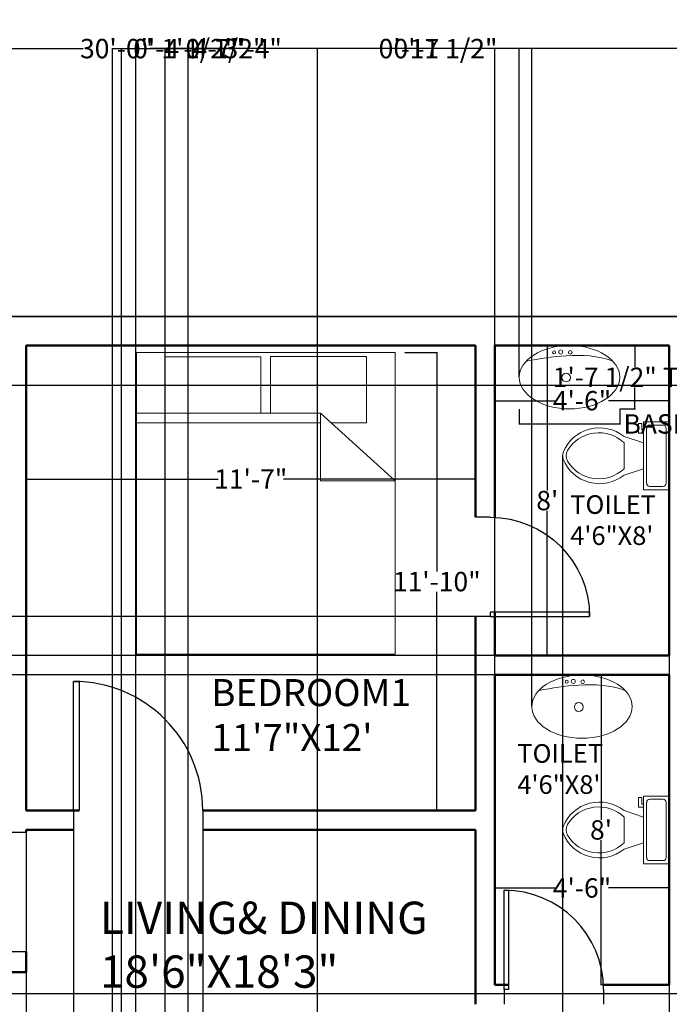
# Model space of a CAD drawing. Units: inches. Extents: x -56 to 545, y -536 to 185.
# Tile 6 of 7: x 144 to 345, y -120 to 185. Entities that reach past the tile are written whole.
import ezdxf

# ---------------------------------------------------------------- set-up
doc = ezdxf.new("R2010")
doc.units = ezdxf.units.IN
doc.header["$MEASUREMENT"] = 0
for name, color, linetype, lineweight in [('A-ANNO-DIMS', 2, 'Continuous', 18), ('A-AREA-IDEN', 4, 'Continuous', 25), ('A-DOOR', 4, 'Continuous', 25), ('A-FLOR-FIXT', 8, 'Continuous', 18), ('A-FURN', 8, 'Continuous', 18), ('A-WALL', 7, 'Continuous', 50), ('C-PROP', 7, 'Continuous', 35)]:
    doc.layers.add(name, color=color, linetype=linetype, lineweight=lineweight)
doc.styles.get("Standard").update_dxf_attribs({"font": 'arial.ttf'})
doc.dimstyles.get("Standard").update_dxf_attribs({"dimtxt": 6, "dimasz": 0.18, "dimexe": 0.18, "dimexo": 0.0625, "dimgap": 0.09, "dimtad": 0, "dimtih": 1, "dimtoh": 1, "dimdec": 0, "dimzin": 0, "dimdsep": 46, "dimlunit": 3, "dimtxsty": 'Standard', "dimcen": 0.09, "dimclrd": 3, "dimclre": 3, "dimclrt": 3, "dimadec": 0, "dimazin": 0, "dimtfac": 1, "dimtdec": 0, "dimtofl": 0, "dimtmove": 0, "dimatfit": 3, "dimfxl": 1, "dimtolj": 1, "dimtzin": 0, "dimarcsym": 0})

# ---------------------------------------------------------------- blocks, each defined once
blk = doc.blocks.new('CAMAKING')
for points in [[(0.8635, 0), (-0.8635, 0)], [(-0.8635, -2.0147), (-0.8635, 0)], [(0.8635, 0), (0.8635, -2.0147)], [(-0.6723, -0.4077), (-0.6723, -0.0281)], [(-0.6723, -0.0281), (-0.0328, -0.0281)], [(-0.0328, -0.0281), (-0.0328, -0.4077)], [(0.6716, -0.027), (0.0319, -0.027)], [(0.0319, -0.027), (0.0319, -0.4077)], [(0.6716, -0.4686), (0.6716, -0.027)], [(0.3645, -0.4056), (-0.8635, -0.4056)], [(0.8635, -0.857), (0.3645, -0.4056)], [(0.3645, -0.4702), (0.3645, -0.4056)], [(-0.8635, -0.4702), (0.3645, -0.4702)], [(0.3645, -0.4702), (0.3645, -0.857)], [(0.4362, -0.4686), (0.6716, -0.4686)], [(0.3645, -0.857), (0.8635, -0.857)], [(0.8635, -2.0147), (-0.8635, -2.0147)]]:
    blk.add_lwpolyline(points)
blk = doc.blocks.new('*U5')
for p, q in [((9.5, -6), (9.5, -2)), ((-10, -8.5), (-8, -8.5)), ((-10, -9.5), (-10, -8.5)), ((-8, -8.5), (-8, -8)), ((-7, -8), (-7, -9.5)), ((-4, -8), (-6, -14)), ((4, -8), (6, -14)), ((-7, -9.5), (-10, -9.5)), ((4, -14), (-4, -14))]:
    blk.add_line(p, q)
blk.add_lwpolyline([(10.5, -8), (10.5, 0), (-10.5, 0), (-10.5, -8)], close=True)
for points in [[(-9.5, -2), (-9.5, -6)], [(8.5, -1), (-8.5, -1)], [(-8.5, -7), (8.5, -7)]]:
    blk.add_lwpolyline(points)
for centre, radius, start, end in [((-8.62, -1.88), 0.884, 81.8699, 188.1301), ((8.62, -1.88), 0.884, 351.8699, 98.1301), ((-8.62, -6.12), 0.884, 171.8699, 278.1301), ((8.62, -6.12), 0.884, 261.8699, 8.1301), ((3.52, -21.58), 12.17, 141.4691, 247.9714), ((4.2, -21.82), 11.33, 136.3677, 238.9468), ((-3.52, -21.58), 12.17, 292.0284, 38.5307), ((-4.2, -21.82), 11.33, 301.053, 43.6321), ((0, -27.88), 4, 245.7318, 294.2682), ((0, -29), 4, 254.8605, 285.1395)]:
    blk.add_arc(centre, radius, start, end)
blk = doc.blocks.new('*U7')
for p, q in [((0, 0), (0, -6)), ((40, 0), (40, -6))]:
    blk.add_line(p, q)
blk.add_lwpolyline([(0, 0), (0, 40), (1.75, 40), (1.75, 0)], close=True)
blk.add_arc((0, 0), 40, 0, 90)
blk = doc.blocks.new('*D26')
at = {"layer": 'A-ANNO-DIMS', "color": 0, "lineweight": -2, "transparency": 16777216}
for p, q in [((146.03, 50.03), (146.03, 42.62)), ((285.03, 50.03), (285.03, 42.62)), ((146.21, 42.8), (205.42, 42.8)), ((284.85, 42.8), (225.65, 42.8))]:
    blk.add_line(p, q, dxfattribs=at)
at = {"layer": 'A-ANNO-DIMS', "color": 0, "transparency": 16777216}
for points in [[(146.21, 42.83), (146.21, 42.77), (146.03, 42.8)], [(284.85, 42.83), (284.85, 42.77), (285.03, 42.8)]]:
    blk.add_solid(points, dxfattribs=at)
at = {"layer": 'Defpoints', "color": 0, "transparency": 16777216}
for p in [(146.03, 50.1), (285.03, 50.1), (285.03, 42.8)]:
    blk.add_point(p, dxfattribs=at)
at = {"layer": 'A-ANNO-DIMS', "color": 0, "transparency": 16777216, "insert": (215.53, 42.8), "char_height": 6, "attachment_point": 5}
blk.add_mtext('\\A1;11\'-7"', dxfattribs=at)
blk = doc.blocks.new('*D27')
at = {"layer": 'A-ANNO-DIMS', "color": 0, "lineweight": -2, "transparency": 16777216}
for p, q in [((263.2, 81.99), (273.28, 81.99)), ((273.1, 81.81), (273.1, 14.23)), ((273.1, -59.66), (273.1, 7.92)), ((263.2, -59.84), (273.28, -59.84))]:
    blk.add_line(p, q, dxfattribs=at)
at = {"layer": 'A-ANNO-DIMS', "color": 0, "transparency": 16777216}
for points in [[(273.07, 81.81), (273.13, 81.81), (273.1, 81.99)], [(273.07, -59.66), (273.13, -59.66), (273.1, -59.84)]]:
    blk.add_solid(points, dxfattribs=at)
at = {"layer": 'Defpoints', "color": 0, "transparency": 16777216}
for p in [(263.14, 81.99), (273.1, 81.99), (263.14, -59.84)]:
    blk.add_point(p, dxfattribs=at)
at = {"layer": 'A-ANNO-DIMS', "color": 0, "transparency": 16777216, "insert": (273.1, 11.07), "char_height": 6, "attachment_point": 5}
blk.add_mtext('\\A1;11\'-10"', dxfattribs=at)
blk = doc.blocks.new('*D28')
at = {"layer": 'A-ANNO-DIMS', "color": 0, "lineweight": -2, "transparency": 16777216}
for p, q in [((291.03, 50.82), (291.03, 67.26)), ((291.21, 67.08), (309.85, 67.08)), ((344.85, 67.08), (326.22, 67.08)), ((345.03, 50.09), (345.03, 67.26))]:
    blk.add_line(p, q, dxfattribs=at)
at = {"layer": 'A-ANNO-DIMS', "color": 0, "transparency": 16777216}
for points in [[(291.21, 67.11), (291.21, 67.05), (291.03, 67.08)], [(344.85, 67.11), (344.85, 67.05), (345.03, 67.08)]]:
    blk.add_solid(points, dxfattribs=at)
at = {"layer": 'Defpoints', "color": 0, "transparency": 16777216}
for p in [(345.03, 67.08), (291.03, 50.76), (345.03, 50.03)]:
    blk.add_point(p, dxfattribs=at)
at = {"layer": 'A-ANNO-DIMS', "color": 0, "transparency": 16777216, "insert": (318.03, 67.08), "char_height": 6, "attachment_point": 5}
blk.add_mtext('\\A1;4\'-6"', dxfattribs=at)
blk = doc.blocks.new('*D29')
at = {"layer": 'A-ANNO-DIMS', "color": 0, "lineweight": -2, "transparency": 16777216}
for p, q in [((335.97, 84.16), (307.11, 84.16)), ((307.29, 83.98), (307.29, 39.31)), ((307.29, -11.66), (307.29, 33.01)), ((335.97, -11.84), (307.11, -11.84))]:
    blk.add_line(p, q, dxfattribs=at)
at = {"layer": 'A-ANNO-DIMS', "color": 0, "transparency": 16777216}
for points in [[(307.26, 83.98), (307.32, 83.98), (307.29, 84.16)], [(307.26, -11.66), (307.32, -11.66), (307.29, -11.84)]]:
    blk.add_solid(points, dxfattribs=at)
at = {"layer": 'Defpoints', "color": 0, "transparency": 16777216}
for p in [(336.04, 84.16), (307.29, -11.84), (336.04, -11.84)]:
    blk.add_point(p, dxfattribs=at)
at = {"layer": 'A-ANNO-DIMS', "color": 0, "transparency": 16777216, "insert": (307.29, 36.16), "char_height": 6, "attachment_point": 5}
blk.add_mtext("\\A1;8'", dxfattribs=at)
blk = doc.blocks.new('*D30')
at = {"layer": 'A-ANNO-DIMS', "color": 0, "lineweight": -2, "transparency": 16777216}
for p, q in [((291.03, -35.73), (291.03, -83.99)), ((345.03, -35.73), (345.03, -83.99)), ((291.21, -83.81), (309.85, -83.81)), ((344.85, -83.81), (326.22, -83.81))]:
    blk.add_line(p, q, dxfattribs=at)
at = {"layer": 'A-ANNO-DIMS', "color": 0, "transparency": 16777216}
for points in [[(291.21, -83.78), (291.21, -83.84), (291.03, -83.81)], [(344.85, -83.78), (344.85, -83.84), (345.03, -83.81)]]:
    blk.add_solid(points, dxfattribs=at)
at = {"layer": 'Defpoints', "color": 0, "transparency": 16777216}
for p in [(291.03, -35.67), (345.03, -35.67), (345.03, -83.81)]:
    blk.add_point(p, dxfattribs=at)
at = {"layer": 'A-ANNO-DIMS', "color": 0, "transparency": 16777216, "insert": (318.03, -83.81), "char_height": 6, "attachment_point": 5}
blk.add_mtext('\\A1;4\'-6"', dxfattribs=at)
blk = doc.blocks.new('*D31')
at = {"layer": 'A-ANNO-DIMS', "color": 0, "lineweight": -2, "transparency": 16777216}
for p, q in [((340.5, -17.84), (323.74, -17.84)), ((323.92, -18.02), (323.92, -62.69)), ((323.92, -113.66), (323.92, -68.99)), ((340.5, -113.84), (323.74, -113.84))]:
    blk.add_line(p, q, dxfattribs=at)
at = {"layer": 'A-ANNO-DIMS', "color": 0, "transparency": 16777216}
for points in [[(323.89, -18.02), (323.95, -18.02), (323.92, -17.84)], [(323.89, -113.66), (323.95, -113.66), (323.92, -113.84)]]:
    blk.add_solid(points, dxfattribs=at)
at = {"layer": 'Defpoints', "color": 0, "transparency": 16777216}
for p in [(340.57, -17.84), (323.92, -113.84), (340.57, -113.84)]:
    blk.add_point(p, dxfattribs=at)
at = {"layer": 'A-ANNO-DIMS', "color": 0, "transparency": 16777216, "insert": (323.92, -65.84), "char_height": 6, "attachment_point": 5}
blk.add_mtext("\\A1;8'", dxfattribs=at)
blk = doc.blocks.new('LAV-OVAL')
for centre, radius in [((-4.76, 7.71), 0.472), ((-2.71, 7.81), 0.633), ((0.21, 7.71), 0.565), ((-1.02, -0.12), 1.35)]:
    blk.add_circle(centre, radius)
blk.add_ellipse((0, 0), major_axis=(-15.53, 0), ratio=0.631418)
blk.add_open_spline([(-13.36, 5), (-9.28, 5.7), (-0.46, 7.23), (8.86, 6.68), (13.36, 5)], degree=3, knots=[0, 0, 0, 0, 12.471835, 26.932887, 26.932887, 26.932887, 26.932887])
blk = doc.blocks.new('*D39')
at = {"layer": 'A-ANNO-DIMS', "color": 3, "lineweight": -2, "transparency": 16777216}
for p, q in [((298.63, 64.49), (298.63, 59.71)), ((329.69, 64.49), (329.69, 59.71)), ((298.81, 59.89), (329.51, 59.89)), ((329.69, 59.89), (329.87, 59.89))]:
    blk.add_line(p, q, dxfattribs=at)
at = {"layer": 'A-ANNO-DIMS', "color": 3, "transparency": 16777216}
for points in [[(298.81, 59.92), (298.81, 59.86), (298.63, 59.89)], [(329.51, 59.92), (329.51, 59.86), (329.69, 59.89)]]:
    blk.add_solid(points, dxfattribs=at)
at = {"layer": 'Defpoints', "color": 0, "transparency": 16777216}
for p in [(298.63, 64.55), (329.69, 64.55), (329.69, 59.89)]:
    blk.add_point(p, dxfattribs=at)
at = {"layer": 'A-ANNO-DIMS', "color": 3, "transparency": 16777216, "insert": (361.86, 59.89), "char_height": 6, "attachment_point": 5}
blk.add_mtext('\\A1;BASIN 2\'-7" TYP.', dxfattribs=at)
blk = doc.blocks.new('*D40')
at = {"layer": 'A-ANNO-DIMS', "color": 3, "lineweight": -2, "transparency": 16777216}
for p, q in [((329.75, 84.16), (334.53, 84.16)), ((334.35, 83.98), (334.35, 77.55)), ((334.35, 64.73), (334.35, 71.16)), ((329.75, 64.55), (334.53, 64.55))]:
    blk.add_line(p, q, dxfattribs=at)
at = {"layer": 'A-ANNO-DIMS', "color": 3, "transparency": 16777216}
for points in [[(334.32, 83.98), (334.38, 83.98), (334.35, 84.16)], [(334.32, 64.73), (334.38, 64.73), (334.35, 64.55)]]:
    blk.add_solid(points, dxfattribs=at)
at = {"layer": 'Defpoints', "color": 0, "transparency": 16777216}
for p in [(329.69, 84.16), (334.35, 84.16), (329.69, 64.55)]:
    blk.add_point(p, dxfattribs=at)
at = {"layer": 'A-ANNO-DIMS', "color": 3, "transparency": 16777216, "insert": (334.35, 74.35), "char_height": 6, "attachment_point": 5}
blk.add_mtext('\\A1;1\'-7 1/2" TYP.', dxfattribs=at)
blk = doc.blocks.new('*D55')
at = {"layer": 'A-ANNO-DIMS', "color": 3, "lineweight": -2, "transparency": 16777216}
for p, q in [((290.97, -11.84), (-38.11, -11.84)), ((-37.93, -12.02), (-37.93, -17.66)), ((290.97, -17.84), (-38.11, -17.84)), ((-37.93, -18.02), (-38.11, -18.02)), ((-37.93, -17.84), (-37.93, -18.02))]:
    blk.add_line(p, q, dxfattribs=at)
at = {"layer": 'A-ANNO-DIMS', "color": 3, "transparency": 16777216}
for points in [[(-37.96, -12.02), (-37.9, -12.02), (-37.93, -11.84)], [(-37.96, -17.66), (-37.9, -17.66), (-37.93, -17.84)]]:
    blk.add_solid(points, dxfattribs=at)
at = {"layer": 'Defpoints', "color": 0, "transparency": 16777216}
for p in [(291.03, -11.84), (-37.93, -17.84), (291.03, -17.84)]:
    blk.add_point(p, dxfattribs=at)
at = {"layer": 'A-ANNO-DIMS', "color": 3, "transparency": 16777216, "insert": (-46.18, -18.02), "char_height": 6, "attachment_point": 5}
blk.add_mtext('\\A1;0\'-6"', dxfattribs=at)
blk = doc.blocks.new('*D61')
at = {"layer": 'A-ANNO-DIMS', "color": 3, "lineweight": -2, "transparency": 16777216}
for p, q in [((175.54, -345.78), (175.54, 176.3)), ((175.72, 176.12), (179.85, 176.12)), ((180.03, -345.78), (180.03, 176.3)), ((180.03, 176.12), (180.21, 176.12))]:
    blk.add_line(p, q, dxfattribs=at)
at = {"layer": 'A-ANNO-DIMS', "color": 3, "transparency": 16777216}
for points in [[(175.72, 176.15), (175.72, 176.09), (175.54, 176.12)], [(179.85, 176.15), (179.85, 176.09), (180.03, 176.12)]]:
    blk.add_solid(points, dxfattribs=at)
at = {"layer": 'Defpoints', "color": 0, "transparency": 16777216}
for p in [(180.03, 176.12), (175.54, -345.84), (180.03, -345.84)]:
    blk.add_point(p, dxfattribs=at)
at = {"layer": 'A-ANNO-DIMS', "color": 3, "transparency": 16777216, "insert": (195.27, 176.12), "char_height": 6, "attachment_point": 5}
blk.add_mtext('\\A1;0\'-4 1/2"', dxfattribs=at)
blk = doc.blocks.new('*D62')
at = {"layer": 'A-ANNO-DIMS', "color": 3, "lineweight": -2, "transparency": 16777216}
for p, q in [((196.14, -419.78), (196.14, 176.3)), ((196.32, 176.12), (208.08, 176.12)), ((235.96, 176.12), (224.21, 176.12)), ((236.14, -419.78), (236.14, 176.3))]:
    blk.add_line(p, q, dxfattribs=at)
at = {"layer": 'A-ANNO-DIMS', "color": 3, "transparency": 16777216}
for points in [[(196.32, 176.15), (196.32, 176.09), (196.14, 176.12)], [(235.96, 176.15), (235.96, 176.09), (236.14, 176.12)]]:
    blk.add_solid(points, dxfattribs=at)
at = {"layer": 'Defpoints', "color": 0, "transparency": 16777216}
for p in [(236.14, 176.12), (196.14, -419.84), (236.14, -419.84)]:
    blk.add_point(p, dxfattribs=at)
at = {"layer": 'A-ANNO-DIMS', "color": 3, "transparency": 16777216, "insert": (216.14, 176.12), "char_height": 6, "attachment_point": 5}
blk.add_mtext('\\A1;3\'-4"', dxfattribs=at)
blk = doc.blocks.new('*D63')
at = {"layer": 'A-ANNO-DIMS', "color": 3, "lineweight": -2, "transparency": 16777216}
for p, q in [((189.03, -410.78), (189.03, 176.3)), ((189.21, 176.12), (195.96, 176.12)), ((196.14, -419.78), (196.14, 176.3)), ((196.14, 176.12), (196.32, 176.12))]:
    blk.add_line(p, q, dxfattribs=at)
at = {"layer": 'A-ANNO-DIMS', "color": 3, "transparency": 16777216}
for points in [[(189.21, 176.15), (189.21, 176.09), (189.03, 176.12)], [(195.96, 176.15), (195.96, 176.09), (196.14, 176.12)]]:
    blk.add_solid(points, dxfattribs=at)
at = {"layer": 'Defpoints', "color": 0, "transparency": 16777216}
for p in [(196.14, 176.12), (189.03, -410.84), (196.14, -419.84)]:
    blk.add_point(p, dxfattribs=at)
at = {"layer": 'A-ANNO-DIMS', "color": 3, "transparency": 16777216, "insert": (204.39, 176.12), "char_height": 6, "attachment_point": 5}
blk.add_mtext('\\A1;0\'-7"', dxfattribs=at)
blk = doc.blocks.new('*D65')
at = {"layer": 'A-ANNO-DIMS', "color": 3, "lineweight": -2, "transparency": 16777216}
for p, q in [((160.69, -65.9), (160.69, -526.99)), ((200.69, -65.9), (200.69, -526.99)), ((160.87, -526.81), (172.63, -526.81)), ((200.51, -526.81), (188.76, -526.81))]:
    blk.add_line(p, q, dxfattribs=at)
at = {"layer": 'A-ANNO-DIMS', "color": 3, "transparency": 16777216}
for points in [[(160.87, -526.78), (160.87, -526.84), (160.69, -526.81)], [(200.51, -526.78), (200.51, -526.84), (200.69, -526.81)]]:
    blk.add_solid(points, dxfattribs=at)
at = {"layer": 'Defpoints', "color": 0, "transparency": 16777216}
for p in [(160.69, -65.84), (200.69, -65.84), (200.69, -526.81)]:
    blk.add_point(p, dxfattribs=at)
at = {"layer": 'A-ANNO-DIMS', "color": 3, "transparency": 16777216, "insert": (180.69, -526.81), "char_height": 6, "attachment_point": 5}
blk.add_mtext('\\A1;3\'-4"', dxfattribs=at)
blk = doc.blocks.new('*D66')
at = {"layer": 'A-ANNO-DIMS', "color": 3, "lineweight": -2, "transparency": 16777216}
for p, q in [((146.03, -65.9), (146.03, -526.99)), ((160.69, -65.9), (160.69, -526.99)), ((146.21, -526.81), (160.51, -526.81)), ((160.69, -526.81), (160.87, -526.81))]:
    blk.add_line(p, q, dxfattribs=at)
at = {"layer": 'A-ANNO-DIMS', "color": 3, "transparency": 16777216}
for points in [[(146.21, -526.78), (146.21, -526.84), (146.03, -526.81)], [(160.51, -526.78), (160.51, -526.84), (160.69, -526.81)]]:
    blk.add_solid(points, dxfattribs=at)
at = {"layer": 'Defpoints', "color": 0, "transparency": 16777216}
for p in [(146.03, -65.84), (160.69, -65.84), (160.69, -526.81)]:
    blk.add_point(p, dxfattribs=at)
at = {"layer": 'A-ANNO-DIMS', "color": 3, "transparency": 16777216, "insert": (175.65, -526.81), "char_height": 6, "attachment_point": 5}
blk.add_mtext('\\A1;1\'-2 1/2"', dxfattribs=at)
blk = doc.blocks.new('*D68')
at = {"layer": 'A-ANNO-DIMS', "color": 3, "lineweight": -2, "transparency": 16777216}
for p, q in [((172.76, -229.78), (172.76, 176.3)), ((172.94, 176.12), (188.85, 176.12)), ((189.03, -229.78), (189.03, 176.3)), ((189.03, 176.12), (189.21, 176.12))]:
    blk.add_line(p, q, dxfattribs=at)
at = {"layer": 'A-ANNO-DIMS', "color": 3, "transparency": 16777216}
for points in [[(172.94, 176.15), (172.94, 176.09), (172.76, 176.12)], [(188.85, 176.15), (188.85, 176.09), (189.03, 176.12)]]:
    blk.add_solid(points, dxfattribs=at)
at = {"layer": 'Defpoints', "color": 0, "transparency": 16777216}
for p in [(189.03, 176.12), (172.76, -229.84), (189.03, -229.84)]:
    blk.add_point(p, dxfattribs=at)
at = {"layer": 'A-ANNO-DIMS', "color": 3, "transparency": 16777216, "insert": (203.99, 176.12), "char_height": 6, "attachment_point": 5}
blk.add_mtext('\\A1;1\'-4 1/2"', dxfattribs=at)
blk = doc.blocks.new('*D70')
at = {"layer": 'A-ANNO-DIMS', "color": 3, "lineweight": -2, "transparency": 16777216}
for p, q in [((421.61, 71.8), (-38.11, 71.8)), ((-37.93, 71.62), (-37.93, -19.2)), ((-37.93, -116.42), (-37.93, -25.59)), ((388.85, -116.6), (-38.11, -116.6))]:
    blk.add_line(p, q, dxfattribs=at)
at = {"layer": 'A-ANNO-DIMS', "color": 3, "transparency": 16777216}
for points in [[(-37.96, 71.62), (-37.9, 71.62), (-37.93, 71.8)], [(-37.96, -116.42), (-37.9, -116.42), (-37.93, -116.6)]]:
    blk.add_solid(points, dxfattribs=at)
at = {"layer": 'Defpoints', "color": 0, "transparency": 16777216}
for p in [(421.67, 71.8), (-37.93, -116.6), (388.91, -116.6)]:
    blk.add_point(p, dxfattribs=at)
at = {"layer": 'A-ANNO-DIMS', "color": 3, "transparency": 16777216, "insert": (-37.93, -22.4), "char_height": 6, "attachment_point": 5}
blk.add_mtext('\\A1;15\'-8 1/2"', dxfattribs=at)
blk = doc.blocks.new('*D72')
at = {"layer": 'A-ANNO-DIMS', "color": 3, "lineweight": -2, "transparency": 16777216}
for p, q in [((289.58, 0.27), (-38.11, 0.27)), ((-37.93, 0.09), (-37.93, -2.63)), ((-37.93, -11.66), (-37.93, -8.94)), ((290.97, -11.84), (-38.11, -11.84))]:
    blk.add_line(p, q, dxfattribs=at)
at = {"layer": 'A-ANNO-DIMS', "color": 3, "transparency": 16777216}
for points in [[(-37.96, 0.09), (-37.9, 0.09), (-37.93, 0.27)], [(-37.96, -11.66), (-37.9, -11.66), (-37.93, -11.84)]]:
    blk.add_solid(points, dxfattribs=at)
at = {"layer": 'Defpoints', "color": 0, "transparency": 16777216}
for p in [(289.64, 0.27), (-37.93, -11.84), (291.03, -11.84)]:
    blk.add_point(p, dxfattribs=at)
at = {"layer": 'A-ANNO-DIMS', "color": 3, "transparency": 16777216, "insert": (-37.93, -5.78), "char_height": 6, "attachment_point": 5}
blk.add_mtext('\\A1;1\'-0"', dxfattribs=at)
blk = doc.blocks.new('*D73')
at = {"layer": 'A-ANNO-DIMS', "color": 3, "lineweight": -2, "transparency": 16777216}
for p, q in [((135.38, 28.1), (135.38, -526.99)), ((140.03, 28.1), (140.03, -526.99)), ((135.56, -526.81), (139.85, -526.81)), ((140.03, -526.81), (140.21, -526.81))]:
    blk.add_line(p, q, dxfattribs=at)
at = {"layer": 'A-ANNO-DIMS', "color": 3, "transparency": 16777216}
for points in [[(135.56, -526.78), (135.56, -526.84), (135.38, -526.81)], [(139.85, -526.78), (139.85, -526.84), (140.03, -526.81)]]:
    blk.add_solid(points, dxfattribs=at)
at = {"layer": 'Defpoints', "color": 0, "transparency": 16777216}
for p in [(135.38, 28.16), (140.03, 28.16), (140.03, -526.81)]:
    blk.add_point(p, dxfattribs=at)
at = {"layer": 'A-ANNO-DIMS', "color": 3, "transparency": 16777216, "insert": (155.27, -526.81), "char_height": 6, "attachment_point": 5}
blk.add_mtext('\\A1;0\'-4 1/2"', dxfattribs=at)
blk = doc.blocks.new('*D81')
at = {"layer": 'A-ANNO-DIMS', "color": 3, "lineweight": -2, "transparency": 16777216}
for p, q in [((345.03, 60.47), (345.03, -526.99)), ((312.03, 49.97), (312.03, -526.99)), ((312.21, -526.81), (320.42, -526.81)), ((344.85, -526.81), (336.65, -526.81))]:
    blk.add_line(p, q, dxfattribs=at)
at = {"layer": 'A-ANNO-DIMS', "color": 3, "transparency": 16777216}
for points in [[(312.21, -526.78), (312.21, -526.84), (312.03, -526.81)], [(344.85, -526.78), (344.85, -526.84), (345.03, -526.81)]]:
    blk.add_solid(points, dxfattribs=at)
at = {"layer": 'Defpoints', "color": 0, "transparency": 16777216}
for p in [(345.03, 60.53), (312.03, 50.03), (312.03, -526.81)]:
    blk.add_point(p, dxfattribs=at)
at = {"layer": 'A-ANNO-DIMS', "color": 3, "transparency": 16777216, "insert": (328.53, -526.81), "char_height": 6, "attachment_point": 5}
blk.add_mtext('\\A1;2\'-9"', dxfattribs=at)
blk = doc.blocks.new('*D88')
at = {"layer": 'A-ANNO-DIMS', "color": 3, "lineweight": -2, "transparency": 16777216}
for p, q in [((291.03, 176.12), (290.85, 176.12)), ((291.03, 84.22), (291.03, 176.3)), ((298.45, 176.12), (291.21, 176.12)), ((298.63, 74.42), (298.63, 176.3))]:
    blk.add_line(p, q, dxfattribs=at)
at = {"layer": 'A-ANNO-DIMS', "color": 3, "transparency": 16777216}
for points in [[(291.21, 176.15), (291.21, 176.09), (291.03, 176.12)], [(298.45, 176.15), (298.45, 176.09), (298.63, 176.12)]]:
    blk.add_solid(points, dxfattribs=at)
at = {"layer": 'Defpoints', "color": 0, "transparency": 16777216}
for p in [(291.03, 176.12), (291.03, 84.16), (298.63, 74.35)]:
    blk.add_point(p, dxfattribs=at)
at = {"layer": 'A-ANNO-DIMS', "color": 3, "transparency": 16777216, "insert": (275.8, 176.12), "char_height": 6, "attachment_point": 5}
blk.add_mtext('\\A1;0\'-7 1/2"', dxfattribs=at)
blk = doc.blocks.new('*D89')
at = {"layer": 'A-ANNO-DIMS', "color": 3, "lineweight": -2, "transparency": 16777216}
for p, q in [((291.03, 176.12), (290.85, 176.12)), ((291.03, -17.78), (291.03, 176.3)), ((302.32, 176.12), (291.21, 176.12)), ((302.5, -27.58), (302.5, 176.3))]:
    blk.add_line(p, q, dxfattribs=at)
at = {"layer": 'A-ANNO-DIMS', "color": 3, "transparency": 16777216}
for points in [[(291.21, 176.15), (291.21, 176.09), (291.03, 176.12)], [(302.32, 176.15), (302.32, 176.09), (302.5, 176.12)]]:
    blk.add_solid(points, dxfattribs=at)
at = {"layer": 'Defpoints', "color": 0, "transparency": 16777216}
for p in [(291.03, 176.12), (291.03, -17.84), (302.5, -27.65)]:
    blk.add_point(p, dxfattribs=at)
at = {"layer": 'A-ANNO-DIMS', "color": 3, "transparency": 16777216, "insert": (273.47, 176.12), "char_height": 6, "attachment_point": 5}
blk.add_mtext('\\A1;0\'-11 1/2"', dxfattribs=at)
blk = doc.blocks.new('*D90')
at = {"layer": 'A-ANNO-DIMS', "color": 3, "lineweight": -2, "transparency": 16777216}
for p, q in [((-5.97, 93.22), (-5.97, 176.3)), ((-5.79, 176.12), (163.64, 176.12)), ((353.85, 176.12), (184.43, 176.12)), ((354.03, 84.22), (354.03, 176.3))]:
    blk.add_line(p, q, dxfattribs=at)
at = {"layer": 'A-ANNO-DIMS', "color": 3, "transparency": 16777216}
for points in [[(-5.79, 176.15), (-5.79, 176.09), (-5.97, 176.12)], [(353.85, 176.15), (353.85, 176.09), (354.03, 176.12)]]:
    blk.add_solid(points, dxfattribs=at)
at = {"layer": 'Defpoints', "color": 0, "transparency": 16777216}
for p in [(354.03, 176.12), (-5.97, 93.16), (354.03, 84.16)]:
    blk.add_point(p, dxfattribs=at)
at = {"layer": 'A-ANNO-DIMS', "color": 3, "transparency": 16777216, "insert": (174.03, 176.12), "char_height": 6, "attachment_point": 5}
blk.add_mtext('\\A1;30\'-0"', dxfattribs=at)

msp = doc.modelspace()

# ---------------------------------------------------------------- linework, layer by layer
at = {"layer": 'A-WALL'}
for p, q in [((146.03, 84.16), (146.03, -59.84)), ((146.03, 84.16), (285.03, 84.16)), ((285.03, 84.16), (285.03, 31)), ((291.03, 84.16), (291.03, 30.97)), ((291.03, 84.16), (345.03, 84.16)), ((345.03, 84.16), (345.03, -11.84)), ((285.03, 0.27), (285.03, -59.84)), ((291.03, 1.62), (291.03, -11.84)), ((291.03, -11.84), (345.03, -11.84)), ((291.03, -17.84), (345.03, -17.84)), ((291.03, -17.84), (291.03, -113.84)), ((345.03, -17.84), (345.03, -113.84)), ((146.03, -59.84), (162.44, -59.84)), ((200.69, -59.84), (285.03, -59.84)), ((146.03, -65.84), (160.69, -65.84)), ((146.03, -65.84), (146.03, -66.51)), ((200.69, -65.84), (285.03, -65.84)), ((285.03, -65.84), (285.03, -119.84)), ((146.03, -103.48), (146.03, -109.84)), ((122.03, -109.84), (146.03, -109.84)), ((291.03, -113.84), (295.31, -113.84)), ((324.66, -113.84), (345.03, -113.84))]:
    msp.add_line(p, q, dxfattribs=at)
at = {"layer": 'C-PROP'}
msp.add_line((-5.97, 93.16), (498.03, 93.16), dxfattribs=at)

# ---------------------------------------------------------------- block references
at = {"layer": 'A-DOOR'}
for p, xscale, yscale, zscale, rotation in [((289.64, 0.27), -0.7680778388986921, 0.7680778388986921, 0.7680778388986921, 270), ((140.49, -103.48), 0.924222506201659, 0.924222506201659, 0.924222506201659, 90)]:
    msp.add_blockref('*U7', p, dxfattribs=dict(at, xscale=xscale, yscale=yscale, zscale=zscale, rotation=rotation))
msp.add_blockref('*U7', (160.69, -59.84), dxfattribs=at)
at = {"layer": 'A-DOOR', "xscale": 0.7680778388986921, "yscale": 0.7680778388986921, "zscale": 0.7680778388986921}
msp.add_blockref('*U7', (293.97, -115.23), dxfattribs=at)
at = {"layer": 'A-FLOR-FIXT'}
for p in [(314.16, 74.35), (318.03, -27.65)]:
    msp.add_blockref('LAV-OVAL', p, dxfattribs=at)
at = {"layer": 'A-FLOR-FIXT', "rotation": 270}
for p in [(345.03, 50.03), (345.03, -65.84)]:
    msp.add_blockref('*U5', p, dxfattribs=at)
at = {"layer": 'A-FURN', "xscale": 46.34928316146463, "yscale": 46.34928316146463, "zscale": 46.34928316146463}
msp.add_blockref('CAMAKING', (220.19, 81.99), dxfattribs=at)

# ---------------------------------------------------------------- texts
at = {"layer": 'A-AREA-IDEN', "attachment_point": 1}
for s, width, gutter_width, insert, char_height in [('{TOILET\\P4\'6"X8\'}', 1091.0728, 28.86, (314.39, 37.8), 5.772), ('{BEDROOM1\\P11\'7"X12\'}', 1579.1545, 41.77, (203.32, -19.13), 8.354), ('{TOILET\\P4\'6"X8\'}', 1091.0728, 28.86, (298.02, -39.28), 5.772), ('{LIVING& DINING \\P18\'6"X18\'3"}', 1091.0728, 28.86, (168.88, -88.05), 10)]:
    msp.add_mtext_dynamic_manual_height_columns(s, width=width, gutter_width=gutter_width, heights=[0], dxfattribs=dict(at, insert=insert, char_height=char_height))

# ---------------------------------------------------------------- dimensions: what is measured, and where the dimension line sits
at = {"layer": 'A-ANNO-DIMS'}
for base, p1, p2, override, picture, middle in [((189.03, 176.12), (172.76, -229.84), (189.03, -229.84), {"dimdec": 1, "dimlfac": 1, "dimrnd": 0, "dimzin": 1, "dimdsep": 46, "dimlunit": 4, "dimfrac": 2}, '*D68', (203.99, 176.12)), ((180.03, 176.12), (175.54, -345.84), (180.03, -345.84), {"dimdec": 1, "dimlfac": 1, "dimrnd": 0, "dimzin": 1, "dimdsep": 46, "dimlunit": 4, "dimfrac": 2}, '*D61', (195.27, 176.12)), ((291.03, 176.12), (302.5, -27.65), (291.03, -17.84), {"dimdec": 1, "dimlfac": 1, "dimrnd": 0, "dimzin": 1, "dimdsep": 46, "dimlunit": 4, "dimfrac": 2}, '*D89', (273.47, 176.12)), ((291.03, 176.12), (298.63, 74.35), (291.03, 84.16), {"dimdec": 1, "dimlfac": 1, "dimrnd": 0, "dimzin": 1, "dimdsep": 46, "dimlunit": 4, "dimfrac": 2}, '*D88', (275.8, 176.12)), ((354.03, 176.12), (-5.97, 93.16), (354.03, 84.16), {"dimdec": 1, "dimlfac": 1, "dimrnd": 0, "dimzin": 1, "dimdsep": 46, "dimlunit": 4, "dimfrac": 2}, '*D90', (174.03, 176.12)), ((196.14, 176.12), (189.03, -410.84), (196.14, -419.84), {"dimdec": 1, "dimlfac": 1, "dimrnd": 0, "dimzin": 1, "dimdsep": 46, "dimlunit": 4, "dimfrac": 2}, '*D63', (204.39, 176.12)), ((236.14, 176.12), (196.14, -419.84), (236.14, -419.84), {"dimdec": 1, "dimlfac": 1, "dimrnd": 0, "dimzin": 1, "dimdsep": 46, "dimlunit": 4, "dimfrac": 2}, '*D62', (216.14, 176.12)), ((345.03, 67.08), (291.03, 50.76), (345.03, 50.03), {"dimclrd": 0, "dimclre": 0, "dimclrt": 0}, '*D28', (318.03, 67.08)), ((312.03, -526.81), (345.03, 60.53), (312.03, 50.03), {"dimdec": 1, "dimlfac": 1, "dimrnd": 0, "dimzin": 1, "dimdsep": 46, "dimlunit": 4, "dimfrac": 2}, '*D81', (328.53, -526.81)), ((285.03, 42.8), (146.03, 50.1), (285.03, 50.1), {"dimclrd": 0, "dimclre": 0, "dimclrt": 0}, '*D26', (215.53, 42.8)), ((140.0343, -526.8056), (135.3838, 28.1594), (140.0343, 28.1594), {"dimdec": 1, "dimlfac": 1, "dimrnd": 0, "dimzin": 1, "dimdsep": 46, "dimlunit": 4, "dimfrac": 2}, '*D73', (155.2695, -526.8056)), ((345.03, -83.81), (291.03, -35.67), (345.03, -35.67), {"dimclrd": 0, "dimclre": 0, "dimclrt": 0}, '*D30', (318.03, -83.81)), ((160.69, -526.81), (146.03, -65.84), (160.69, -65.84), {"dimdec": 1, "dimlfac": 1, "dimrnd": 0, "dimzin": 1, "dimdsep": 46, "dimlunit": 4, "dimfrac": 2}, '*D66', (175.65, -526.81)), ((200.69, -526.81), (160.69, -65.84), (200.69, -65.84), {"dimdec": 1, "dimlfac": 1, "dimrnd": 0, "dimzin": 1, "dimdsep": 46, "dimlunit": 4, "dimfrac": 2}, '*D65', (180.69, -526.81))]:
    dim = msp.add_linear_dim(base=base, p1=p1, p2=p2, dimstyle='Standard', override=override, dxfattribs=at)
    dim.commit()
    dim.dimension.update_dxf_attribs({"geometry": picture, "text_midpoint": middle})
dim = msp.add_linear_dim(base=(334.35, 84.16), p1=(329.69, 64.55), p2=(329.69, 84.16), angle=90, text='<> TYP.', dimstyle='Standard', override={"dimdec": 1, "dimlfac": 1, "dimrnd": 0, "dimzin": 1, "dimdsep": 46, "dimlunit": 4, "dimfrac": 2}, dxfattribs=at)
dim.commit()
dim.dimension.update_dxf_attribs({"geometry": '*D40', "text_midpoint": (334.35, 74.35)})
for base, p1, p2, override, picture, middle in [((307.29, -11.84), (336.04, 84.16), (336.04, -11.84), {"dimclrd": 0, "dimclre": 0, "dimclrt": 0}, '*D29', (307.29, 36.16)), ((273.1, 81.99), (263.14, -59.84), (263.14, 81.99), {"dimclrd": 0, "dimclre": 0, "dimclrt": 0}, '*D27', (273.1, 11.07)), ((-37.93, -116.6), (421.67, 71.8), (388.91, -116.6), {"dimdec": 1, "dimlfac": 1, "dimrnd": 0, "dimzin": 1, "dimdsep": 46, "dimlunit": 4, "dimfrac": 2}, '*D70', (-37.93, -22.4)), ((-37.93, -11.84), (289.64, 0.27), (291.03, -11.84), {"dimdec": 1, "dimlfac": 1, "dimrnd": 0, "dimzin": 1, "dimdsep": 46, "dimlunit": 4, "dimfrac": 2}, '*D72', (-37.93, -5.78)), ((-37.93, -17.84), (291.03, -11.84), (291.03, -17.84), {"dimdec": 1, "dimlfac": 1, "dimrnd": 0, "dimzin": 1, "dimdsep": 46, "dimlunit": 4, "dimfrac": 2}, '*D55', (-46.18, -18.02)), ((323.92, -113.84), (340.57, -17.84), (340.57, -113.84), {"dimclrd": 0, "dimclre": 0, "dimclrt": 0}, '*D31', (323.92, -65.84))]:
    dim = msp.add_linear_dim(base=base, p1=p1, p2=p2, angle=90, dimstyle='Standard', override=override, dxfattribs=at)
    dim.commit()
    dim.dimension.update_dxf_attribs({"geometry": picture, "text_midpoint": middle})
dim = msp.add_linear_dim(base=(329.69, 59.89), p1=(298.63, 64.55), p2=(329.69, 64.55), text='BASIN <> TYP.', dimstyle='Standard', override={"dimdec": 1, "dimlfac": 1, "dimrnd": 0, "dimzin": 1, "dimdsep": 46, "dimlunit": 4, "dimfrac": 2}, dxfattribs=at)
dim.commit()
dim.dimension.update_dxf_attribs({"geometry": '*D39', "text_midpoint": (361.86, 59.89)})

doc.saveas('drawing.dxf')
